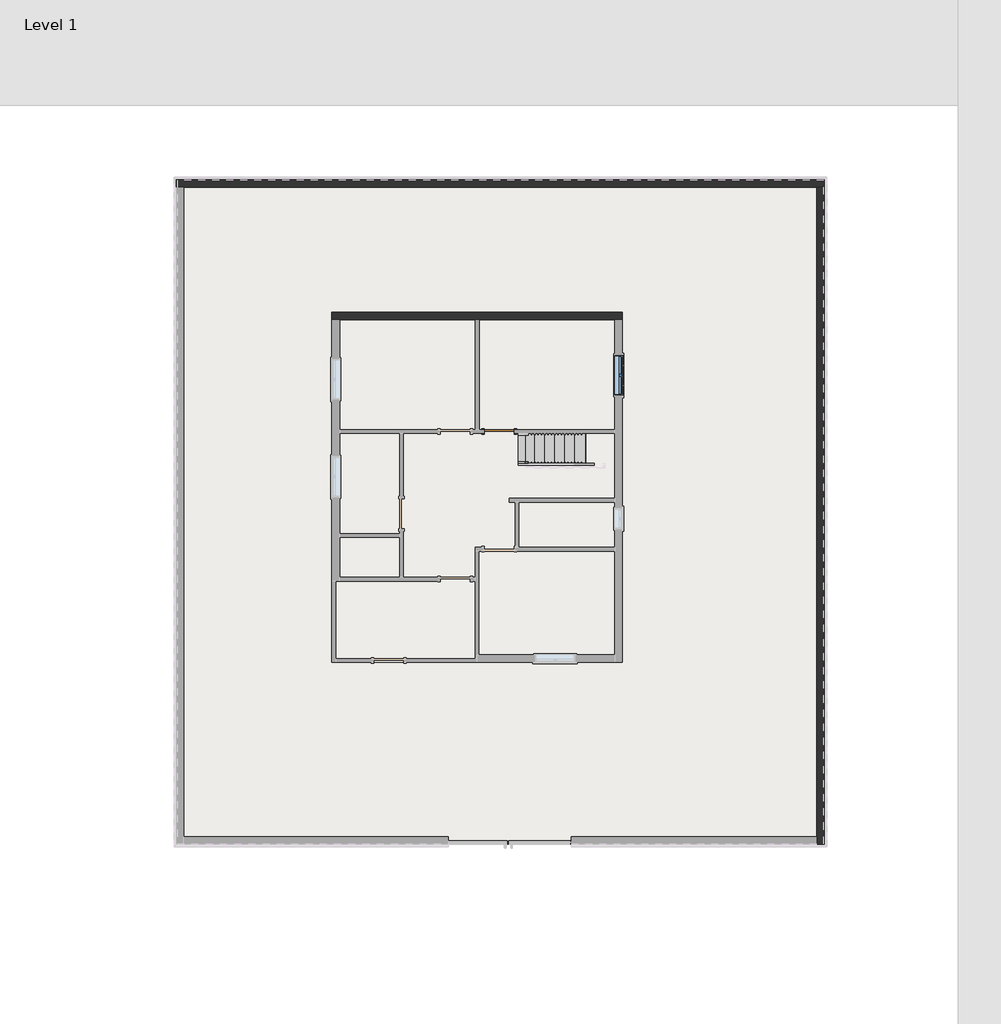
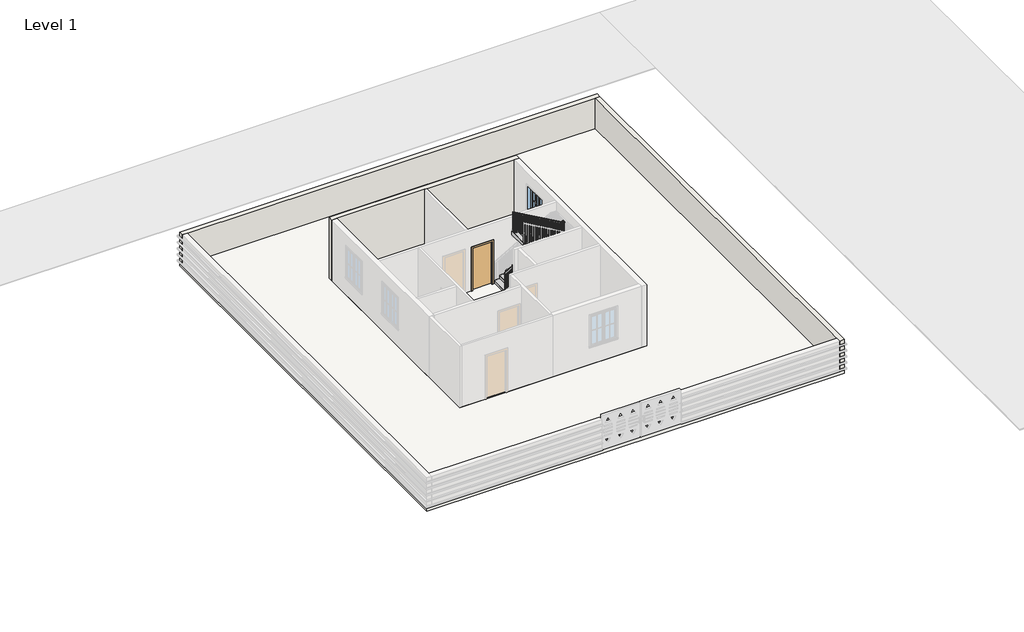
# One storey, part 2 of 3: 3 walls, 2 slabs, 1 door, 1 railing, 1 stair flight, 1 window.
"""IFC4 building model written with IfcOpenShell, lengths in millimetres."""

from ifc_helpers import new_model, si_unit, frame, origin, place, context, project, spatial, polyline, outline, extrude, faceted_brep, transform, mapped, element, save
from components import door_305aa2a5, stair_flight_fa6bf0c5, window_8377141f

model = new_model("IFC4")

# Units and contexts
model_context = context("Model", 3, world=origin())
ifc_project = project(units=[si_unit("LENGTHUNIT", "METRE", prefix="MILLI")], contexts=[model_context])

# Site, building, storey
site = spatial("IfcSite", under=ifc_project)
building = spatial("IfcBuilding", under=site)
storey = spatial("IfcBuildingStorey", under=building, Name="Level 1", Elevation=0.0)

# Door
placement = place(None, origin())
door_shape = door_305aa2a5(model_context)
element("IfcDoor", 1, ObjectType="Single-Flush : 36\" x 84\"", at=placement, inside=storey, context=model_context, shape_type="MappedRepresentation", body=[
    mapped(door_shape, transform((8001.0, 9251.95, 0.0), x_axis=(-1.0, 0.0, 0.0), y_axis=(0.0, -1.0, 0.0), z_axis=(0.0, 0.0, 1.0))),
])

# Railing
element("IfcRailing", 2, ObjectType="Handrail - Rectangular", at=placement, inside=storey, context=model_context, shape_type="SolidModel", body=[
    faceted_brep([(8572.5, 8331.2, 1083.7333333), (8572.5, 8331.2, 1025.0853937), (8572.5, 8280.4, 1025.0853937), (8572.5, 8280.4, 1083.7333333), (11137.9, 8331.2, 2563.7717949), (11188.7, 8331.2, 2534.4315475), (11188.7, 8280.4, 2534.4315475), (11137.9, 8280.4, 2563.7717949), (11137.9, 8331.2, 2607.7333333), (11188.7, 8331.2, 2556.9333333), (11188.7, 8280.4, 2556.9333333), (11137.9, 8280.4, 2607.7333333), (11264.9, 8331.2, 2607.7333333), (11264.9, 8331.2, 2556.9333333), (11214.1, 8280.4, 2556.9333333), (11214.1, 8280.4, 2607.7333333), (11264.9, 8204.2, 2607.7333333), (11264.9, 8153.4, 2556.9333333), (11214.1, 8153.4, 2556.9333333), (11214.1, 8204.2, 2607.7333333), (11264.9, 8204.2, 2820.3007092), (11264.9, 8153.4, 2769.5007092), (11214.1, 8153.4, 2769.5007092), (11214.1, 8204.2, 2820.3007092), (11264.9, 8077.2, 2820.3007092), (11264.9, 8077.2, 2769.5007092), (11214.1, 8128.0, 2769.5007092), (11214.1, 8128.0, 2820.3007092), (11137.9, 8077.2, 2820.3007092), (11124.4925101, 8077.2, 2769.5007092), (11124.4925101, 8128.0, 2769.5007092), (11137.9, 8128.0, 2820.3007092), (8826.5, 8077.2, 4131.7333333), (8826.5, 8128.0, 4131.7333333), (8826.5, 8128.0, 4073.3262469), (8826.5, 8077.2, 4073.3262469)], [[[0, 1, 2, 3]], [[1, 0, 4, 5]], [[2, 1, 5, 6]], [[3, 2, 6, 7]], [[0, 3, 7, 4]], [[5, 4, 8, 9]], [[6, 5, 9, 10]], [[7, 6, 10, 11]], [[4, 7, 11, 8]], [[9, 8, 12, 13]], [[10, 9, 13, 14]], [[11, 10, 14, 15]], [[8, 11, 15, 12]], [[13, 12, 16, 17]], [[14, 13, 17, 18]], [[15, 14, 18, 19]], [[12, 15, 19, 16]], [[17, 16, 20, 21]], [[18, 17, 21, 22]], [[19, 18, 22, 23]], [[16, 19, 23, 20]], [[21, 20, 24, 25]], [[22, 21, 25, 26]], [[23, 22, 26, 27]], [[20, 23, 27, 24]], [[25, 24, 28, 29]], [[26, 25, 29, 30]], [[27, 26, 30, 31]], [[24, 27, 31, 28]], [[32, 33, 34, 35]], [[29, 28, 32, 35]], [[30, 29, 35, 34]], [[31, 30, 34, 33]], [[28, 31, 33, 32]]]),
    extrude(outline(polyline([(4024.687949, 8912.225), (4035.4964596, 8893.175), (3048.0, 8893.175), (3048.0, 8912.225), (4024.687949, 8912.225)])), frame((0.0, 8093.075, 0.0), z_axis=(0.0, 1.0, 0.0), x_axis=(0.0, 0.0, 1.0)), (0.0, 0.0, 1.0), 19.05),
    extrude(outline(polyline([(3967.0425589, 9013.825), (3977.8510696, 8994.775), (3048.0, 8994.775), (3048.0, 9013.825), (3967.0425589, 9013.825)])), frame((0.0, 8093.075, 0.0), z_axis=(0.0, 1.0, 0.0), x_axis=(0.0, 0.0, 1.0)), (0.0, 0.0, 1.0), 19.05),
    extrude(outline(polyline([(3909.3971689, 9115.425), (3920.2056795, 9096.375), (2878.6666667, 9096.375), (2878.6666667, 9115.425), (3909.3971689, 9115.425)])), frame((0.0, 8093.075, 0.0), z_axis=(0.0, 1.0, 0.0), x_axis=(0.0, 0.0, 1.0)), (0.0, 0.0, 1.0), 19.05),
    extrude(outline(polyline([(3851.7517788, 9217.025), (3862.5602894, 9197.975), (2878.6666667, 9197.975), (2878.6666667, 9217.025), (3851.7517788, 9217.025)])), frame((0.0, 8093.075, 0.0), z_axis=(0.0, 1.0, 0.0), x_axis=(0.0, 0.0, 1.0)), (0.0, 0.0, 1.0), 19.05),
    extrude(outline(polyline([(3794.0517398, 9318.625), (3805.0421244, 9299.575), (2878.6666667, 9299.575), (2878.6666667, 9318.625), (3794.0517398, 9318.625)])), frame((0.0, 8093.075, 0.0), z_axis=(0.0, 1.0, 0.0), x_axis=(0.0, 0.0, 1.0)), (0.0, 0.0, 1.0), 19.05),
    extrude(outline(polyline([(3736.4609986, 9420.225), (3747.2695093, 9401.175), (2709.3333333, 9401.175), (2709.3333333, 9420.225), (3736.4609986, 9420.225)])), frame((0.0, 8093.075, 0.0), z_axis=(0.0, 1.0, 0.0), x_axis=(0.0, 0.0, 1.0)), (0.0, 0.0, 1.0), 19.05),
    extrude(outline(polyline([(3678.8156086, 9521.825), (3689.6241192, 9502.775), (2709.3333333, 9502.775), (2709.3333333, 9521.825), (3678.8156086, 9521.825)])), frame((0.0, 8093.075, 0.0), z_axis=(0.0, 1.0, 0.0), x_axis=(0.0, 0.0, 1.0)), (0.0, 0.0, 1.0), 19.05),
    extrude(outline(polyline([(3621.1702185, 9623.425), (3631.9787291, 9604.375), (2709.3333333, 9604.375), (2709.3333333, 9623.425), (3621.1702185, 9623.425)])), frame((0.0, 8093.075, 0.0), z_axis=(0.0, 1.0, 0.0), x_axis=(0.0, 0.0, 1.0)), (0.0, 0.0, 1.0), 19.05),
    extrude(outline(polyline([(3563.5248284, 9725.025), (3574.3333391, 9705.975), (2540.0, 9705.975), (2540.0, 9725.025), (3563.5248284, 9725.025)])), frame((0.0, 8093.075, 0.0), z_axis=(0.0, 1.0, 0.0), x_axis=(0.0, 0.0, 1.0)), (0.0, 0.0, 1.0), 19.05),
    extrude(outline(polyline([(3505.8794384, 9826.625), (3516.687949, 9807.575), (2540.0, 9807.575), (2540.0, 9826.625), (3505.8794384, 9826.625)])), frame((0.0, 8093.075, 0.0), z_axis=(0.0, 1.0, 0.0), x_axis=(0.0, 0.0, 1.0)), (0.0, 0.0, 1.0), 19.05),
    extrude(outline(polyline([(3448.2340483, 9928.225), (3459.0425589, 9909.175), (2540.0, 9909.175), (2540.0, 9928.225), (3448.2340483, 9928.225)])), frame((0.0, 8093.075, 0.0), z_axis=(0.0, 1.0, 0.0), x_axis=(0.0, 0.0, 1.0)), (0.0, 0.0, 1.0), 19.05),
    extrude(outline(polyline([(3390.5886582, 10029.825), (3401.3971689, 10010.775), (2370.6666667, 10010.775), (2370.6666667, 10029.825), (3390.5886582, 10029.825)])), frame((0.0, 8093.075, 0.0), z_axis=(0.0, 1.0, 0.0), x_axis=(0.0, 0.0, 1.0)), (0.0, 0.0, 1.0), 19.05),
    extrude(outline(polyline([(3332.9432681, 10131.425), (3343.7517788, 10112.375), (2370.6666667, 10112.375), (2370.6666667, 10131.425), (3332.9432681, 10131.425)])), frame((0.0, 8093.075, 0.0), z_axis=(0.0, 1.0, 0.0), x_axis=(0.0, 0.0, 1.0)), (0.0, 0.0, 1.0), 19.05),
    extrude(outline(polyline([(3275.2978781, 10233.025), (3286.1063887, 10213.975), (2370.6666667, 10213.975), (2370.6666667, 10233.025), (3275.2978781, 10233.025)])), frame((0.0, 8093.075, 0.0), z_axis=(0.0, 1.0, 0.0), x_axis=(0.0, 0.0, 1.0)), (0.0, 0.0, 1.0), 19.05),
    extrude(outline(polyline([(3217.652488, 10334.625), (3228.4609986, 10315.575), (2201.3333333, 10315.575), (2201.3333333, 10334.625), (3217.652488, 10334.625)])), frame((0.0, 8093.075, 0.0), z_axis=(0.0, 1.0, 0.0), x_axis=(0.0, 0.0, 1.0)), (0.0, 0.0, 1.0), 19.05),
    extrude(outline(polyline([(3160.0070979, 10436.225), (3170.8156086, 10417.175), (2201.3333333, 10417.175), (2201.3333333, 10436.225), (3160.0070979, 10436.225)])), frame((0.0, 8093.075, 0.0), z_axis=(0.0, 1.0, 0.0), x_axis=(0.0, 0.0, 1.0)), (0.0, 0.0, 1.0), 19.05),
    extrude(outline(polyline([(3102.3617079, 10537.825), (3113.1702185, 10518.775), (2201.3333333, 10518.775), (2201.3333333, 10537.825), (3102.3617079, 10537.825)])), frame((0.0, 8093.075, 0.0), z_axis=(0.0, 1.0, 0.0), x_axis=(0.0, 0.0, 1.0)), (0.0, 0.0, 1.0), 19.05),
    extrude(outline(polyline([(3044.7163178, 10639.425), (3055.5248284, 10620.375), (2032.0, 10620.375), (2032.0, 10639.425), (3044.7163178, 10639.425)])), frame((0.0, 8093.075, 0.0), z_axis=(0.0, 1.0, 0.0), x_axis=(0.0, 0.0, 1.0)), (0.0, 0.0, 1.0), 19.05),
    extrude(outline(polyline([(2987.0709277, 10741.025), (2997.8794384, 10721.975), (2032.0, 10721.975), (2032.0, 10741.025), (2987.0709277, 10741.025)])), frame((0.0, 8093.075, 0.0), z_axis=(0.0, 1.0, 0.0), x_axis=(0.0, 0.0, 1.0)), (0.0, 0.0, 1.0), 19.05),
    extrude(outline(polyline([(2929.4255377, 10842.625), (2940.2340483, 10823.575), (2032.0, 10823.575), (2032.0, 10842.625), (2929.4255377, 10842.625)])), frame((0.0, 8093.075, 0.0), z_axis=(0.0, 1.0, 0.0), x_axis=(0.0, 0.0, 1.0)), (0.0, 0.0, 1.0), 19.05),
    extrude(outline(polyline([(2871.7801476, 10944.225), (2882.5886582, 10925.175), (1862.6666667, 10925.175), (1862.6666667, 10944.225), (2871.7801476, 10944.225)])), frame((0.0, 8093.075, 0.0), z_axis=(0.0, 1.0, 0.0), x_axis=(0.0, 0.0, 1.0)), (0.0, 0.0, 1.0), 19.05),
    extrude(outline(polyline([(2814.1347575, 11045.825), (2824.9432681, 11026.775), (1862.6666667, 11026.775), (1862.6666667, 11045.825), (2814.1347575, 11045.825)])), frame((0.0, 8093.075, 0.0), z_axis=(0.0, 1.0, 0.0), x_axis=(0.0, 0.0, 1.0)), (0.0, 0.0, 1.0), 19.05),
    extrude(outline(polyline([(2756.4893674, 11147.425), (2767.2978781, 11128.375), (1862.6666667, 11128.375), (1862.6666667, 11147.425), (2756.4893674, 11147.425)])), frame((0.0, 8093.075, 0.0), z_axis=(0.0, 1.0, 0.0), x_axis=(0.0, 0.0, 1.0)), (0.0, 0.0, 1.0), 19.05),
    extrude(outline(polyline([(11229.975, 8213.725), (11249.025, 8213.725), (11249.025, 8194.675), (11229.975, 8194.675), (11229.975, 8213.725)])), frame((0.0, 0.0, 1693.3333333), z_axis=(0.0, 0.0, 1.0), x_axis=(1.0, 0.0, 0.0)), (0.0, 0.0, 1.0), 863.6),
    extrude(outline(polyline([(11204.575, 8296.275), (11204.575, 8315.325), (11223.625, 8315.325), (11223.625, 8296.275), (11204.575, 8296.275)])), frame((0.0, 0.0, 1693.3333333), z_axis=(0.0, 0.0, 1.0), x_axis=(1.0, 0.0, 0.0)), (0.0, 0.0, 1.0), 863.6),
    extrude(outline(polyline([(2495.9652013, 11122.025), (2484.9748167, 11102.975), (1524.0, 11102.975), (1524.0, 11122.025), (2495.9652013, 11122.025)])), frame((0.0, 8296.275, 0.0), z_axis=(0.0, 1.0, 0.0), x_axis=(0.0, 0.0, 1.0)), (0.0, 0.0, 1.0), 19.05),
    extrude(outline(polyline([(2437.3498167, 11020.425), (2426.3594321, 11001.375), (1524.0, 11001.375), (1524.0, 11020.425), (2437.3498167, 11020.425)])), frame((0.0, 8296.275, 0.0), z_axis=(0.0, 1.0, 0.0), x_axis=(0.0, 0.0, 1.0)), (0.0, 0.0, 1.0), 19.05),
    extrude(outline(polyline([(2378.7344321, 10918.825), (2367.7440475, 10899.775), (1524.0, 10899.775), (1524.0, 10918.825), (2378.7344321, 10918.825)])), frame((0.0, 8296.275, 0.0), z_axis=(0.0, 1.0, 0.0), x_axis=(0.0, 0.0, 1.0)), (0.0, 0.0, 1.0), 19.05),
    extrude(outline(polyline([(2320.1190475, 10817.225), (2309.1286629, 10798.175), (1354.6666667, 10798.175), (1354.6666667, 10817.225), (2320.1190475, 10817.225)])), frame((0.0, 8296.275, 0.0), z_axis=(0.0, 1.0, 0.0), x_axis=(0.0, 0.0, 1.0)), (0.0, 0.0, 1.0), 19.05),
    extrude(outline(polyline([(2261.5036629, 10715.625), (2250.5132783, 10696.575), (1354.6666667, 10696.575), (1354.6666667, 10715.625), (2261.5036629, 10715.625)])), frame((0.0, 8296.275, 0.0), z_axis=(0.0, 1.0, 0.0), x_axis=(0.0, 0.0, 1.0)), (0.0, 0.0, 1.0), 19.05),
    extrude(outline(polyline([(2202.8882783, 10614.025), (2191.8978937, 10594.975), (1354.6666667, 10594.975), (1354.6666667, 10614.025), (2202.8882783, 10614.025)])), frame((0.0, 8296.275, 0.0), z_axis=(0.0, 1.0, 0.0), x_axis=(0.0, 0.0, 1.0)), (0.0, 0.0, 1.0), 19.05),
    extrude(outline(polyline([(2144.2728937, 10512.425), (2133.282509, 10493.375), (1185.3333333, 10493.375), (1185.3333333, 10512.425), (2144.2728937, 10512.425)])), frame((0.0, 8296.275, 0.0), z_axis=(0.0, 1.0, 0.0), x_axis=(0.0, 0.0, 1.0)), (0.0, 0.0, 1.0), 19.05),
    extrude(outline(polyline([(2085.657509, 10410.825), (2074.6671244, 10391.775), (1185.3333333, 10391.775), (1185.3333333, 10410.825), (2085.657509, 10410.825)])), frame((0.0, 8296.275, 0.0), z_axis=(0.0, 1.0, 0.0), x_axis=(0.0, 0.0, 1.0)), (0.0, 0.0, 1.0), 19.05),
    extrude(outline(polyline([(2027.0421244, 10309.225), (2016.0517398, 10290.175), (1185.3333333, 10290.175), (1185.3333333, 10309.225), (2027.0421244, 10309.225)])), frame((0.0, 8296.275, 0.0), z_axis=(0.0, 1.0, 0.0), x_axis=(0.0, 0.0, 1.0)), (0.0, 0.0, 1.0), 19.05),
    extrude(outline(polyline([(1968.4267398, 10207.625), (1957.4363552, 10188.575), (1016.0, 10188.575), (1016.0, 10207.625), (1968.4267398, 10207.625)])), frame((0.0, 8296.275, 0.0), z_axis=(0.0, 1.0, 0.0), x_axis=(0.0, 0.0, 1.0)), (0.0, 0.0, 1.0), 19.05),
    extrude(outline(polyline([(1909.8113552, 10106.025), (1898.8209706, 10086.975), (1016.0, 10086.975), (1016.0, 10106.025), (1909.8113552, 10106.025)])), frame((0.0, 8296.275, 0.0), z_axis=(0.0, 1.0, 0.0), x_axis=(0.0, 0.0, 1.0)), (0.0, 0.0, 1.0), 19.05),
    extrude(outline(polyline([(1851.1959706, 10004.425), (1840.205586, 9985.375), (1016.0, 9985.375), (1016.0, 10004.425), (1851.1959706, 10004.425)])), frame((0.0, 8296.275, 0.0), z_axis=(0.0, 1.0, 0.0), x_axis=(0.0, 0.0, 1.0)), (0.0, 0.0, 1.0), 19.05),
    extrude(outline(polyline([(1792.580586, 9902.825), (1781.5902013, 9883.775), (846.6666667, 9883.775), (846.6666667, 9902.825), (1792.580586, 9902.825)])), frame((0.0, 8296.275, 0.0), z_axis=(0.0, 1.0, 0.0), x_axis=(0.0, 0.0, 1.0)), (0.0, 0.0, 1.0), 19.05),
    extrude(outline(polyline([(1733.9652013, 9801.225), (1722.9748167, 9782.175), (846.6666667, 9782.175), (846.6666667, 9801.225), (1733.9652013, 9801.225)])), frame((0.0, 8296.275, 0.0), z_axis=(0.0, 1.0, 0.0), x_axis=(0.0, 0.0, 1.0)), (0.0, 0.0, 1.0), 19.05),
    extrude(outline(polyline([(1675.3498167, 9699.625), (1664.3594321, 9680.575), (846.6666667, 9680.575), (846.6666667, 9699.625), (1675.3498167, 9699.625)])), frame((0.0, 8296.275, 0.0), z_axis=(0.0, 1.0, 0.0), x_axis=(0.0, 0.0, 1.0)), (0.0, 0.0, 1.0), 19.05),
    extrude(outline(polyline([(1616.7344321, 9598.025), (1605.7440475, 9578.975), (677.3333333, 9578.975), (677.3333333, 9598.025), (1616.7344321, 9598.025)])), frame((0.0, 8296.275, 0.0), z_axis=(0.0, 1.0, 0.0), x_axis=(0.0, 0.0, 1.0)), (0.0, 0.0, 1.0), 19.05),
    extrude(outline(polyline([(1558.1190475, 9496.425), (1547.1286629, 9477.375), (677.3333333, 9477.375), (677.3333333, 9496.425), (1558.1190475, 9496.425)])), frame((0.0, 8296.275, 0.0), z_axis=(0.0, 1.0, 0.0), x_axis=(0.0, 0.0, 1.0)), (0.0, 0.0, 1.0), 19.05),
    extrude(outline(polyline([(1499.5036629, 9394.825), (1488.5132783, 9375.775), (677.3333333, 9375.775), (677.3333333, 9394.825), (1499.5036629, 9394.825)])), frame((0.0, 8296.275, 0.0), z_axis=(0.0, 1.0, 0.0), x_axis=(0.0, 0.0, 1.0)), (0.0, 0.0, 1.0), 19.05),
    extrude(outline(polyline([(1440.8882783, 9293.225), (1429.8978937, 9274.175), (508.0, 9274.175), (508.0, 9293.225), (1440.8882783, 9293.225)])), frame((0.0, 8296.275, 0.0), z_axis=(0.0, 1.0, 0.0), x_axis=(0.0, 0.0, 1.0)), (0.0, 0.0, 1.0), 19.05),
    extrude(outline(polyline([(1382.2728937, 9191.625), (1371.282509, 9172.575), (508.0, 9172.575), (508.0, 9191.625), (1382.2728937, 9191.625)])), frame((0.0, 8296.275, 0.0), z_axis=(0.0, 1.0, 0.0), x_axis=(0.0, 0.0, 1.0)), (0.0, 0.0, 1.0), 19.05),
    extrude(outline(polyline([(1323.657509, 9090.025), (1312.6671244, 9070.975), (508.0, 9070.975), (508.0, 9090.025), (1323.657509, 9090.025)])), frame((0.0, 8296.275, 0.0), z_axis=(0.0, 1.0, 0.0), x_axis=(0.0, 0.0, 1.0)), (0.0, 0.0, 1.0), 19.05),
    extrude(outline(polyline([(1265.0421244, 8988.425), (1254.0517398, 8969.375), (338.6666667, 8969.375), (338.6666667, 8988.425), (1265.0421244, 8988.425)])), frame((0.0, 8296.275, 0.0), z_axis=(0.0, 1.0, 0.0), x_axis=(0.0, 0.0, 1.0)), (0.0, 0.0, 1.0), 19.05),
    extrude(outline(polyline([(1206.4267398, 8886.825), (1195.4363552, 8867.775), (338.6666667, 8867.775), (338.6666667, 8886.825), (1206.4267398, 8886.825)])), frame((0.0, 8296.275, 0.0), z_axis=(0.0, 1.0, 0.0), x_axis=(0.0, 0.0, 1.0)), (0.0, 0.0, 1.0), 19.05),
    extrude(outline(polyline([(1147.8113552, 8785.225), (1136.8209706, 8766.175), (169.3333333, 8766.175), (169.3333333, 8785.225), (1147.8113552, 8785.225)])), frame((0.0, 8296.275, 0.0), z_axis=(0.0, 1.0, 0.0), x_axis=(0.0, 0.0, 1.0)), (0.0, 0.0, 1.0), 19.05),
    extrude(outline(polyline([(1089.1959706, 8683.625), (1078.205586, 8664.575), (169.3333333, 8664.575), (169.3333333, 8683.625), (1089.1959706, 8683.625)])), frame((0.0, 8296.275, 0.0), z_axis=(0.0, 1.0, 0.0), x_axis=(0.0, 0.0, 1.0)), (0.0, 0.0, 1.0), 19.05),
    extrude(outline(polyline([(11229.975, 8112.125), (11249.025, 8112.125), (11249.025, 8093.075), (11229.975, 8093.075), (11229.975, 8112.125)])), frame((0.0, 0.0, 1693.3333333), z_axis=(0.0, 0.0, 1.0), x_axis=(1.0, 0.0, 0.0)), (0.0, 0.0, 1.0), 1076.1673759),
    extrude(outline(polyline([(11229.975, 8296.275), (11229.975, 8315.325), (11249.025, 8315.325), (11249.025, 8296.275), (11229.975, 8296.275)])), frame((0.0, 0.0, 1693.3333333), z_axis=(0.0, 0.0, 1.0), x_axis=(1.0, 0.0, 0.0)), (0.0, 0.0, 1.0), 863.6),
    extrude(outline(polyline([(4062.5177362, 8845.55), (4073.3262469, 8826.5), (3048.0, 8826.5), (3048.0, 8845.55), (4062.5177362, 8845.55)])), frame((0.0, 8093.075, 0.0), z_axis=(0.0, 1.0, 0.0), x_axis=(0.0, 0.0, 1.0)), (0.0, 0.0, 1.0), 19.05),
    extrude(outline(polyline([(1036.0757783, 8591.55), (1025.0853937, 8572.5), (169.3333333, 8572.5), (169.3333333, 8591.55), (1036.0757783, 8591.55)])), frame((0.0, 8296.275, 0.0), z_axis=(0.0, 1.0, 0.0), x_axis=(0.0, 0.0, 1.0)), (0.0, 0.0, 1.0), 19.05),
])

# Slabs
element("IfcSlab", 3, ObjectType="Generic - 12\"", at=placement, inside=storey, context=model_context, shape_type="SweptSolid", body=[
    extrude(outline(polyline([(11747.5, 12890.5), (11747.5, 2222.5), (2908.3, 2222.5), (2908.3, 12890.5), (11747.5, 12890.5)])), frame((0.0, 0.0, -152.4), z_axis=(0.0, 0.0, 1.0), x_axis=(1.0, 0.0, 0.0)), (0.0, 0.0, 1.0), 152.4),
])
element("IfcSlab", 4, ObjectType="Generic - 12\"", at=placement, inside=storey, context=model_context, shape_type="SweptSolid", body=[
    extrude(outline(polyline([(17900.8586384, 16924.129251), (17900.8586384, -3319.670749), (-1834.9413616, -3319.670749), (-1834.9413616, 16924.129251), (17900.8586384, 16924.129251)])), frame((0.0, 0.0, -152.4), z_axis=(0.0, 0.0, 1.0), x_axis=(1.0, 0.0, 0.0)), (0.0, 0.0, 1.0), 152.4),
])

# Stair flight
stair_flight_shape = stair_flight_fa6bf0c5(model_context)
element("IfcStairFlight", 5, ObjectType="2\" Tread 1\" Nosing 1/4\" Riser", at=placement, inside=storey, context=model_context, shape_type="MappedRepresentation", body=[
    mapped(stair_flight_shape, transform((0.0, 0.0, 0.0), x_axis=(1.0, 0.0, 0.0), y_axis=(0.0, 1.0, 0.0), z_axis=(0.0, 0.0, 1.0))),
])

# Walls
element("IfcWall", 6, ObjectType="Generic - 8\"", at=placement, inside=storey, context=model_context, shape_type="Brep", body=[
    faceted_brep([(2908.3, 12661.9, 0.0), (3136.9, 12661.9, 0.0), (7277.1, 12661.9, 0.0), (7391.4, 12661.9, 0.0), (11518.9, 12661.9, 0.0), (11747.5, 12661.9, 0.0), (11747.5, 12661.9, 3048.0), (11518.9, 12661.9, 3048.0), (7391.4, 12661.9, 3048.0), (7277.1, 12661.9, 3048.0), (3136.9, 12661.9, 3048.0), (2908.3, 12661.9, 3048.0), (2908.3, 12890.5, 0.0), (2908.3, 12890.5, 3048.0), (11747.5, 12890.5, 3048.0), (11747.5, 12890.5, 0.0)], [[[0, 1, 2, 3, 4, 5, 6, 7, 8, 9, 10, 11]], [[12, 13, 14, 15]], [[5, 4, 3, 2, 1, 0, 12, 15]], [[6, 5, 15, 14]], [[0, 11, 13, 12]], [[11, 10, 9, 8, 7, 6, 14, 13]]]),
])
element("IfcWall", 7, ObjectType="Generic - 8\"", at=placement, inside=storey, context=model_context, shape_type="Brep", body=[
    faceted_brep([(-1834.9413616, 16695.529251, 0.0), (-1606.3413616, 16695.529251, 0.0), (17672.2586384, 16695.529251, 0.0), (17900.8586384, 16695.529251, 0.0), (17900.8586384, 16695.529251, 50.8), (17875.4586384, 16695.529251, 50.8), (17875.4586384, 16695.529251, 118.5333333), (17900.8586384, 16695.529251, 118.5333333), (17900.8586384, 16695.529251, 355.6), (17875.4586384, 16695.529251, 355.6), (17875.4586384, 16695.529251, 423.3333333), (17900.8586384, 16695.529251, 423.3333333), (17900.8586384, 16695.529251, 660.4), (17875.4586384, 16695.529251, 660.4), (17875.4586384, 16695.529251, 728.1333333), (17900.8586384, 16695.529251, 728.1333333), (17900.8586384, 16695.529251, 965.2), (17875.4586384, 16695.529251, 965.2), (17875.4586384, 16695.529251, 1032.9333333), (17900.8586384, 16695.529251, 1032.9333333), (17900.8586384, 16695.529251, 1270.0), (17875.4586384, 16695.529251, 1270.0), (17875.4586384, 16695.529251, 1337.7333333), (17900.8586384, 16695.529251, 1337.7333333), (17900.8586384, 16695.529251, 1524.0), (17672.2586384, 16695.529251, 1524.0), (-1606.3413616, 16695.529251, 1524.0), (-1834.9413616, 16695.529251, 1524.0), (-1834.9413616, 16695.529251, 1337.7333333), (-1809.5413616, 16695.529251, 1337.7333333), (-1809.5413616, 16695.529251, 1270.0), (-1834.9413616, 16695.529251, 1270.0), (-1834.9413616, 16695.529251, 1032.9333333), (-1809.5413616, 16695.529251, 1032.9333333), (-1809.5413616, 16695.529251, 965.2), (-1834.9413616, 16695.529251, 965.2), (-1834.9413616, 16695.529251, 728.1333333), (-1809.5413616, 16695.529251, 728.1333333), (-1809.5413616, 16695.529251, 660.4), (-1834.9413616, 16695.529251, 660.4), (-1834.9413616, 16695.529251, 423.3333333), (-1809.5413616, 16695.529251, 423.3333333), (-1809.5413616, 16695.529251, 355.6), (-1834.9413616, 16695.529251, 355.6), (-1834.9413616, 16695.529251, 118.5333333), (-1809.5413616, 16695.529251, 118.5333333), (-1809.5413616, 16695.529251, 50.8), (-1834.9413616, 16695.529251, 50.8), (17900.8586384, 16924.129251, 0.0), (-1834.9413616, 16924.129251, 0.0), (-1834.9413616, 16924.129251, 50.8), (17900.8586384, 16924.129251, 50.8), (-1834.9413616, 16924.129251, 1524.0), (17900.8586384, 16924.129251, 1524.0), (17900.8586384, 16924.129251, 1337.7333333), (-1834.9413616, 16924.129251, 1337.7333333), (17900.8586384, 16924.129251, 118.5333333), (-1834.9413616, 16924.129251, 118.5333333), (-1834.9413616, 16924.129251, 355.6), (17900.8586384, 16924.129251, 355.6), (17900.8586384, 16924.129251, 423.3333333), (-1834.9413616, 16924.129251, 423.3333333), (-1834.9413616, 16924.129251, 660.4), (17900.8586384, 16924.129251, 660.4), (17900.8586384, 16924.129251, 728.1333333), (-1834.9413616, 16924.129251, 728.1333333), (-1834.9413616, 16924.129251, 965.2), (17900.8586384, 16924.129251, 965.2), (17900.8586384, 16924.129251, 1032.9333333), (-1834.9413616, 16924.129251, 1032.9333333), (-1834.9413616, 16924.129251, 1270.0), (17900.8586384, 16924.129251, 1270.0), (17875.4586384, 16898.729251, 118.5333333), (-1809.5413616, 16898.729251, 118.5333333), (-1809.5413616, 16898.729251, 50.8), (17875.4586384, 16898.729251, 50.8), (17875.4586384, 16898.729251, 423.3333333), (-1809.5413616, 16898.729251, 423.3333333), (-1809.5413616, 16898.729251, 355.6), (17875.4586384, 16898.729251, 355.6), (17875.4586384, 16898.729251, 728.1333333), (-1809.5413616, 16898.729251, 728.1333333), (-1809.5413616, 16898.729251, 660.4), (17875.4586384, 16898.729251, 660.4), (17875.4586384, 16898.729251, 1032.9333333), (-1809.5413616, 16898.729251, 1032.9333333), (-1809.5413616, 16898.729251, 965.2), (17875.4586384, 16898.729251, 965.2), (17875.4586384, 16898.729251, 1337.7333333), (-1809.5413616, 16898.729251, 1337.7333333), (-1809.5413616, 16898.729251, 1270.0), (17875.4586384, 16898.729251, 1270.0)], [[[0, 1, 2, 3, 4, 5, 6, 7, 8, 9, 10, 11, 12, 13, 14, 15, 16, 17, 18, 19, 20, 21, 22, 23, 24, 25, 26, 27, 28, 29, 30, 31, 32, 33, 34, 35, 36, 37, 38, 39, 40, 41, 42, 43, 44, 45, 46, 47]], [[48, 49, 50, 51]], [[52, 53, 54, 55]], [[56, 57, 58, 59]], [[60, 61, 62, 63]], [[64, 65, 66, 67]], [[68, 69, 70, 71]], [[3, 48, 51, 4]], [[53, 24, 23, 54]], [[7, 56, 59, 8]], [[11, 60, 63, 12]], [[15, 64, 67, 16]], [[19, 68, 71, 20]], [[27, 52, 55, 28]], [[49, 0, 47, 50]], [[57, 44, 43, 58]], [[61, 40, 39, 62]], [[65, 36, 35, 66]], [[69, 32, 31, 70]], [[3, 2, 1, 0, 49, 48]], [[27, 26, 25, 24, 53, 52]], [[72, 73, 45, 44, 57, 56, 7, 6]], [[74, 75, 5, 4, 51, 50, 47, 46]], [[73, 74, 46, 45]], [[73, 72, 75, 74]], [[75, 72, 6, 5]], [[76, 77, 41, 40, 61, 60, 11, 10]], [[78, 79, 9, 8, 59, 58, 43, 42]], [[77, 78, 42, 41]], [[77, 76, 79, 78]], [[79, 76, 10, 9]], [[80, 81, 37, 36, 65, 64, 15, 14]], [[82, 83, 13, 12, 63, 62, 39, 38]], [[81, 82, 38, 37]], [[81, 80, 83, 82]], [[83, 80, 14, 13]], [[84, 85, 33, 32, 69, 68, 19, 18]], [[86, 87, 17, 16, 67, 66, 35, 34]], [[85, 86, 34, 33]], [[85, 84, 87, 86]], [[87, 84, 18, 17]], [[88, 89, 29, 28, 55, 54, 23, 22]], [[90, 91, 21, 20, 71, 70, 31, 30]], [[89, 90, 30, 29]], [[89, 88, 91, 90]], [[91, 88, 22, 21]]]),
])
element("IfcWall", 8, ObjectType="Generic - 8\"", at=placement, inside=storey, context=model_context, shape_type="Brep", body=[
    faceted_brep([(17672.2586384, 16695.529251, 0.0), (17672.2586384, -3091.070749, 0.0), (17672.2586384, -3319.670749, 0.0), (17672.2586384, -3319.670749, 50.8), (17672.2586384, -3294.270749, 50.8), (17672.2586384, -3294.270749, 118.5333333), (17672.2586384, -3319.670749, 118.5333333), (17672.2586384, -3319.670749, 355.6), (17672.2586384, -3294.270749, 355.6), (17672.2586384, -3294.270749, 423.3333333), (17672.2586384, -3319.670749, 423.3333333), (17672.2586384, -3319.670749, 660.4), (17672.2586384, -3294.270749, 660.4), (17672.2586384, -3294.270749, 728.1333333), (17672.2586384, -3319.670749, 728.1333333), (17672.2586384, -3319.670749, 965.2), (17672.2586384, -3294.270749, 965.2), (17672.2586384, -3294.270749, 1032.9333333), (17672.2586384, -3319.670749, 1032.9333333), (17672.2586384, -3319.670749, 1270.0), (17672.2586384, -3294.270749, 1270.0), (17672.2586384, -3294.270749, 1337.7333333), (17672.2586384, -3319.670749, 1337.7333333), (17672.2586384, -3319.670749, 1524.0), (17672.2586384, -3091.070749, 1524.0), (17672.2586384, 16695.529251, 1524.0), (17900.8586384, -3319.670749, 0.0), (17900.8586384, 16695.529251, 0.0), (17900.8586384, 16695.529251, 50.8), (17900.8586384, -3319.670749, 50.8), (17900.8586384, 16695.529251, 1524.0), (17900.8586384, -3319.670749, 1524.0), (17900.8586384, -3319.670749, 1337.7333333), (17900.8586384, 16695.529251, 1337.7333333), (17900.8586384, -3319.670749, 118.5333333), (17900.8586384, 16695.529251, 118.5333333), (17900.8586384, 16695.529251, 355.6), (17900.8586384, -3319.670749, 355.6), (17900.8586384, -3319.670749, 423.3333333), (17900.8586384, 16695.529251, 423.3333333), (17900.8586384, 16695.529251, 660.4), (17900.8586384, -3319.670749, 660.4), (17900.8586384, -3319.670749, 728.1333333), (17900.8586384, 16695.529251, 728.1333333), (17900.8586384, 16695.529251, 965.2), (17900.8586384, -3319.670749, 965.2), (17900.8586384, -3319.670749, 1032.9333333), (17900.8586384, 16695.529251, 1032.9333333), (17900.8586384, 16695.529251, 1270.0), (17900.8586384, -3319.670749, 1270.0), (17875.4586384, 16695.529251, 1337.7333333), (17875.4586384, 16695.529251, 1270.0), (17875.4586384, 16695.529251, 1032.9333333), (17875.4586384, 16695.529251, 965.2), (17875.4586384, 16695.529251, 728.1333333), (17875.4586384, 16695.529251, 660.4), (17875.4586384, 16695.529251, 423.3333333), (17875.4586384, 16695.529251, 355.6), (17875.4586384, 16695.529251, 118.5333333), (17875.4586384, 16695.529251, 50.8), (17875.4586384, -3294.270749, 118.5333333), (17875.4586384, -3294.270749, 50.8), (17875.4586384, -3294.270749, 423.3333333), (17875.4586384, -3294.270749, 355.6), (17875.4586384, -3294.270749, 728.1333333), (17875.4586384, -3294.270749, 660.4), (17875.4586384, -3294.270749, 1032.9333333), (17875.4586384, -3294.270749, 965.2), (17875.4586384, -3294.270749, 1337.7333333), (17875.4586384, -3294.270749, 1270.0)], [[[0, 1, 2, 3, 4, 5, 6, 7, 8, 9, 10, 11, 12, 13, 14, 15, 16, 17, 18, 19, 20, 21, 22, 23, 24, 25]], [[26, 27, 28, 29]], [[30, 31, 32, 33]], [[34, 35, 36, 37]], [[38, 39, 40, 41]], [[42, 43, 44, 45]], [[46, 47, 48, 49]], [[2, 1, 0, 27, 26]], [[25, 24, 23, 31, 30]], [[0, 25, 30, 33, 50, 51, 48, 47, 52, 53, 44, 43, 54, 55, 40, 39, 56, 57, 36, 35, 58, 59, 28, 27]], [[2, 26, 29, 3]], [[31, 23, 22, 32]], [[6, 34, 37, 7]], [[10, 38, 41, 11]], [[14, 42, 45, 15]], [[18, 46, 49, 19]], [[5, 60, 58, 35, 34, 6]], [[59, 61, 4, 3, 29, 28]], [[60, 61, 59, 58]], [[61, 60, 5, 4]], [[9, 62, 56, 39, 38, 10]], [[57, 63, 8, 7, 37, 36]], [[62, 63, 57, 56]], [[63, 62, 9, 8]], [[13, 64, 54, 43, 42, 14]], [[55, 65, 12, 11, 41, 40]], [[64, 65, 55, 54]], [[65, 64, 13, 12]], [[17, 66, 52, 47, 46, 18]], [[53, 67, 16, 15, 45, 44]], [[66, 67, 53, 52]], [[67, 66, 17, 16]], [[21, 68, 50, 33, 32, 22]], [[51, 69, 20, 19, 49, 48]], [[68, 69, 51, 50]], [[69, 68, 21, 20]]]),
])

# Window
window_shape = window_8377141f(model_context)
element("IfcWindow", 9, ObjectType="Window-Casement-Double : 48\" x 60\"", at=placement, inside=storey, context=model_context, shape_type="MappedRepresentation", body=[
    mapped(window_shape, transform((11633.2, 10961.6875, 0.0), x_axis=(0.0, -1.0, 0.0), y_axis=(1.0, 0.0, 0.0), z_axis=(0.0, 0.0, 1.0))),
])

save(model, "model.ifc")

# Revit data of these elements
# Type "Single-Flush : 36\" x 84\""
#   Type Mark = "1"
#   Construction Type Id = "MDOOR"
#   Assembly Code = "C1020"
#   Analytic Construction = "Metal"
#   Thickness = 0' - 2"
#   Heat Transfer Coefficient (U) = 0.651978 BTU/(h·ft²·°F)
#   Height = 7' - 0"
#   Trim Projection Ext = 0' - 1"
#   Trim Projection Int = 0' - 1"
#   Trim Width = 0' - 3"
#   Width = 3' - 0"
#   Define Thermal Properties by = 1
#   Define Thermal Properties by = 1
#   Door Material = Door - Panel
#   Frame Material = Door - Frame
#   Visual Light Transmittance = 0
#   Solar Heat Gain Coefficient = 0
#   Function = (empty or 0)
#   Wall Closure = (empty or 0)
# Type "Handrail - Rectangular"
#   Assembly Code = "C2010400"
#   built-in parameter 1008612 = 0.0416667 (stored number, unit not read)
#   built-in parameter 1008611 = 0.0416667 (stored number, unit not read)
#   built-in parameter 1008609 = 0.333333 (stored number, unit not read)
#   built-in parameter 1008604 = 0.166667 (stored number, unit not read)
#   built-in parameter 1008603 = 0.166667 (stored number, unit not read)
#   Railing Height = 3' - 0"
#   built-in parameter 1008630 = 2
#   built-in parameter 1008610 = 2
#   built-in parameter 1008618 = Baluster - Square : 3/4"
# Type "Generic - 12\""
#   Assembly Code = "B1010"
#   Function = 0
#   Layers, outside or top first: 0' - 6" no material (function 1)
# Type "Generic - 8\""
#   Assembly Code = "B2010"
#   Layers, outside or top first: 0' - 9" "Parking Stripe" (function 1)
# Type "Window-Casement-Double : 48\" x 60\""
#   Type Mark = "17"
#   Fire Rating = "0.5h"
#   Assembly Code = "B2020100"
#   Analytic Construction = "Double glazing - domestic"
#   Frame Extension [instance default] = 0' - 0 1/4"
#   Window Inset [instance default] = 0' - 0"
#   Wall Thickness [instance default] = 0' - 6"
#   Interior Wall Closure [instance default] = 0' - 2 1/4"
#   Half Width = 2' - 0"
#   Visual Light Transmittance = 0.81
#   Thermal Resistance (R) = 1.8146 (h·ft²·°F)/BTU
#   Solar Heat Gain Coefficient = 0.76
#   Rough Width = 4' - 0 1/2"
#   Rough Height = 5' - 0 1/2"
#   Height = 5' - 0"
#   Heat Transfer Coefficient (U) = 0.5511 BTU/(h·ft²·°F)
#   Exterior Wall Closure [instance default] = 0' - 1 1/4"
#   Extension Jamb [instance default] = 0' - 2 1/4"
#   Default Sill Height = 3' - 0"
#   Width = 4' - 0"
#   Define Thermal Properties by = 0
#   Muntin Visibility = yes
#   Interior Trim Visibility [instance default] = yes
#   Exterior Trim Visibility [instance default] = yes
#   Extension Jamb Visibility [instance default] = yes
#   Interior Trim Material = Wood - Stained
#   Muntin Pattern = Muntin Pattern_2x2 : Muntin Pattern_2x2
#   Interior Trim = Trim-Window-Interior-Flat : Picture Frame
#   Interior Frame Material = Wood - Stained
#   Glass Panel Material = Glass
#   Exterior Trim Material = Clad - White
#   Exterior Trim = Trim-Window-Exterior-Flat : with Sill
#   Exterior Frame Material = Clad - White
#   Wall Closure = (empty or 0)
# Element 1 (IfcDoor, "Single-Flush : 36\" x 84\"")
#   Phase Created = New Construction
#   Materials on its faces: "Door - Frame", "Door - Panel"
# Element 2 (IfcRailing, "Handrail - Rectangular")
#   Phase Created = New Construction
# Element 3 (IfcSlab, "Generic - 12\"")
#   Height Offset From Level = 0' - 0"
#   Phase Created = New Construction
#   Materials on its faces: "Default Floor"
# Element 4 (IfcSlab, "Generic - 12\"")
#   Height Offset From Level = 0' - 0"
#   Phase Created = New Construction
#   Materials on its faces: "Clad - White", "Default Floor", "Cherry"
# Element 5 (IfcStairFlight, "2\" Tread 1\" Nosing 1/4\" Riser")
#   Phase Created = New Construction
# Element 6 (IfcWall, "Generic - 8\"")
#   Top Offset = 0' - 0"
#   Base Offset = 0' - 0"
#   Unconnected Height = 10' - 0"
#   wall height = 10' - 0"
#   Phase Created = New Construction
#   Base Constraint = Level 1
#   Materials on its faces: "Parking Stripe", "Cherry"
# Elements 7, 8 (IfcWall, "Generic - 8\"")
#   Top Offset = 0' - 0"
#   Base Offset = 0' - 0"
#   Unconnected Height = 5' - 0"
#   wall height = 5' - 0"
#   Phase Created = New Construction
#   Base Constraint = Level 1
#   Materials on its faces: "Parking Stripe", "Clad - White", "Cherry"
# Element 9 (IfcWindow, "Window-Casement-Double : 48\" x 60\"")
#   Mark = "4"
#   Window Inset = 0' - 0"
#   Interior Wall Closure = 0' - 2 1/4"
#   Frame Extension = 0' - 0 1/4"
#   Exterior Wall Closure = 0' - 1 1/4"
#   Interior Trim Visibility = yes
#   Exterior Trim Visibility = yes
#   Phase Created = New Construction
#   Materials on its faces: "Wood - Stained", "Glass", "Clad - White"
# Materials
#   "Door - Panel": class "Wood", colour RGB 210 159 95, transparency 0, Cost = 0
#   "Door - Frame": colour RGB 118 70 51, transparency 0, Cost = 0
#   "Parking Stripe": class "Paint", colour RGB 250 250 91, transparency 0, Cost = 0
#   "Wood - Stained": class "Wood", colour RGB 224 178 126, transparency 0, Cost = 0
#   "Glass": class "Glass", colour RGB 0 128 192, transparency 0.75, Description = "Soda Lime Glass", Cost = 0
#   "Clad - White": class "Wood", colour RGB 242 242 238, transparency 0, Cost = 0
#   "Default Floor": colour RGB 128 128 128, transparency 0, Cost = 0
#   "Cherry": class "Wood", colour RGB 226 177 128, transparency 0, Description = "Prunus Serotina", Cost = 0
